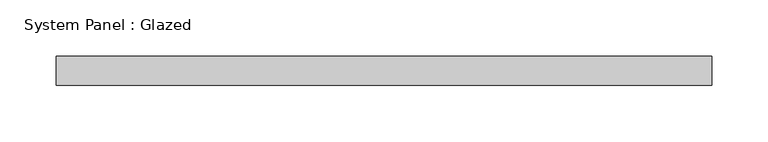
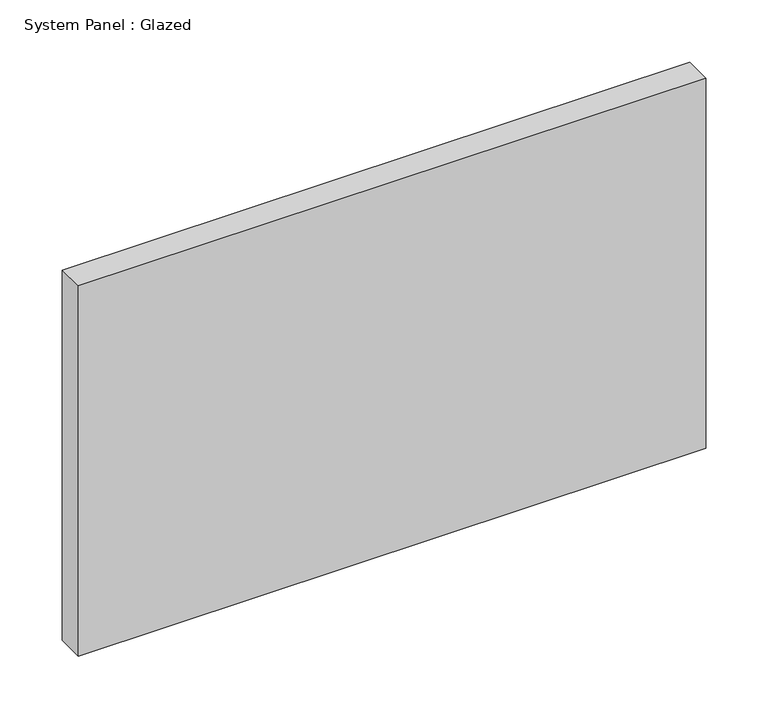
"""IFC4 building model written with IfcOpenShell, lengths in millimetres: plate geometry, System Panel : Glazed."""

from ifc_helpers import new_model, si_unit, origin, origin_with_axes, place, context, project, spatial, polyline, outline, extrude, source, transform, mapped, element, save


def system_panel_glazed_5c6b2ea2(model_context):
    return source(origin(), model_context, "Body", "SweptSolid", [
        extrude(outline(polyline([(289.9833333, 19.05), (-289.9833333, 19.05), (-289.9833333, 44.45), (289.9833333, 44.45), (289.9833333, 19.05)])), origin_with_axes(), (0.0, 0.0, 1.0), 361.95),
    ])


if __name__ == "__main__":
    model = new_model("IFC4")
    model_context = context("Model", 3, world=origin())
    ifc_project = project(units=[si_unit("LENGTHUNIT", "METRE", prefix="MILLI")], contexts=[model_context])
    site = spatial("IfcSite", under=ifc_project)
    building = spatial("IfcBuilding", under=site)
    placement = place(None, origin())
    system_panel_glazed_shape = system_panel_glazed_5c6b2ea2(model_context)
    element("IfcPlate", 1, ObjectType="System Panel : Glazed", at=placement, inside=building, context=model_context, shape_type="MappedRepresentation", body=[
        mapped(system_panel_glazed_shape, transform((0.0, 0.0, 0.0), x_axis=(1.0, 0.0, 0.0), y_axis=(0.0, 1.0, 0.0), z_axis=(0.0, 0.0, 1.0))),
    ])
    save(model, "model.ifc")

# Revit data of these elements
# Type "System Panel : Glazed"
#   Construction Type Id = "GSP4R"
#   Analytic Construction = "1/8 in Pilkington single glazing"
#   Visual Light Transmittance = 0.9
#   Solar Heat Gain Coefficient = 0.86
#   Heat Transfer Coefficient (U) = 1.18115 BTU/(h·ft²·°F)
# Element 1 (IfcPlate, "System Panel : Glazed")
#   Materials on its faces: "Glass"
# Materials
#   "Glass": class "Glass", colour RGB 0 128 192, transparency 0.75, Description = "Soda Lime Glass", Cost = 0
